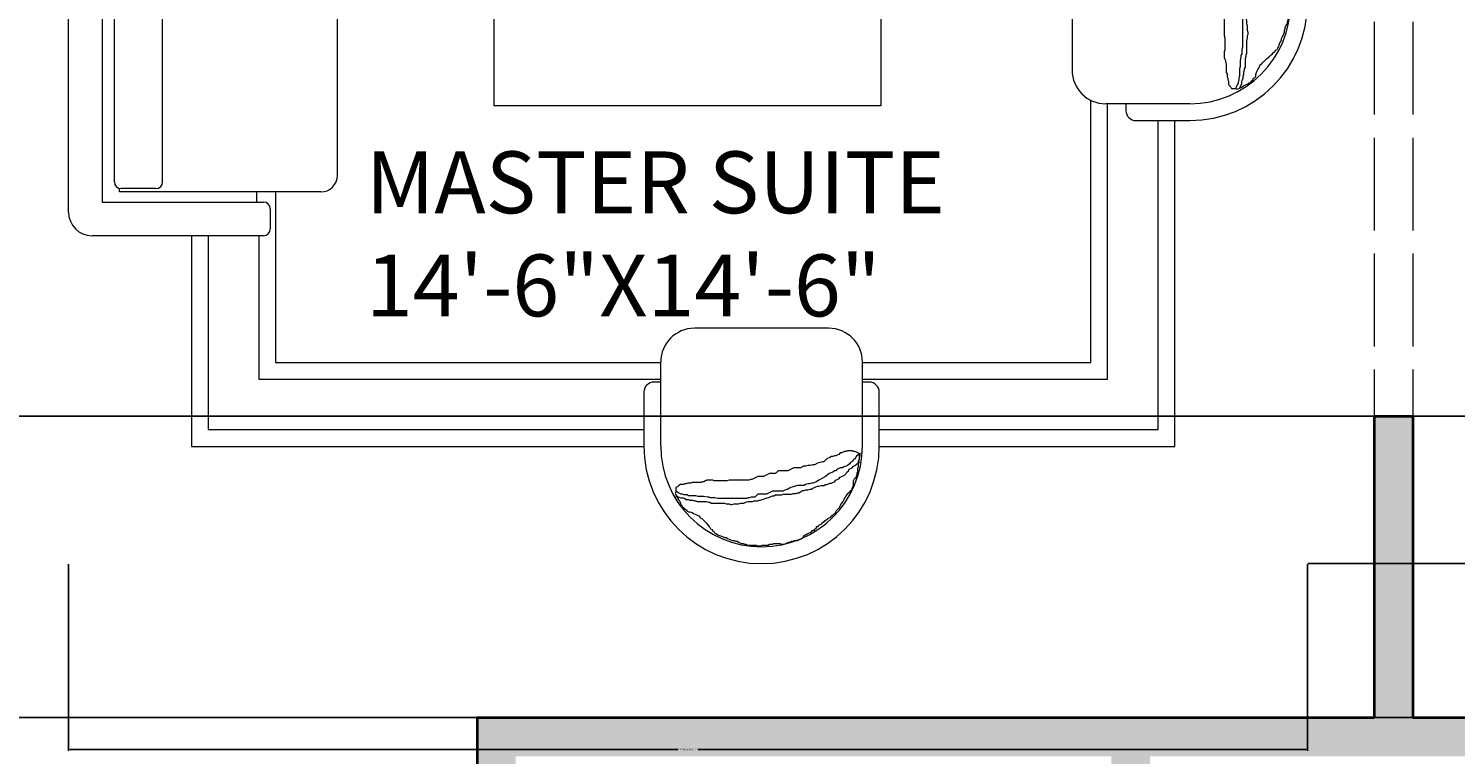
# Model space of a CAD drawing. Units: inches. Extents: x 2330 to 3943, y 1763 to 3461.
# Tile 28 of 40: x 3097 to 3281, y 2975 to 3069. Entities that reach past the tile are written whole.
import ezdxf

# ---------------------------------------------------------------- set-up
doc = ezdxf.new("R2010")
doc.units = ezdxf.units.IN
doc.linetypes.add('ACAD_ISO02W100', pattern=[15, 12, -3])
for name, color, linetype, lineweight in [('A-ANNO-DIMS', 2, 'Continuous', 18), ('A-AREA-IDEN', 7, 'Continuous', 18), ('A-FURN', 8, 'Continuous', 13), ('A-WALL', 7, 'Continuous', 40), ('A-WALL-OVHD', 7, 'ACAD_ISO02W100', 18), ('A-WALL-PATT', 252, 'Continuous', 13)]:
    doc.layers.add(name, color=color, linetype=linetype, lineweight=lineweight)
doc.styles.get("Standard").update_dxf_attribs({"font": 'arial.ttf'})
doc.dimstyles.get("Standard").update_dxf_attribs({"dimtxt": 0.18, "dimasz": 0.18, "dimexe": 0.18, "dimexo": 0.0625, "dimgap": 0.09, "dimtad": 0, "dimtih": 1, "dimtoh": 1, "dimdec": 4, "dimzin": 0, "dimdsep": 46, "dimtxsty": 'Standard', "dimcen": 0.09, "dimadec": 0, "dimazin": 0, "dimtfac": 1, "dimtdec": 4, "dimtofl": 0, "dimtmove": 0, "dimatfit": 3, "dimfxl": 1, "dimtolj": 1, "dimtzin": 0, "dimarcsym": 0})

# ---------------------------------------------------------------- blocks, each defined once
blk = doc.blocks.new('A$C78064EA7')
for p, q in [((932.1, 3320.6), (2792.1, 3320.6)), ((862.1, 2740.6), (862.1, 3250.6)), ((2862.1, 3250.6), (2862.1, 2740.6)), ((962.1, 3220.6), (962.1, 2740.6)), ((2762.1, 3220.6), (962.1, 3220.6)), ((1022.1, 3184.3), (1532.1, 3184.3)), ((1612.1, 3184.3), (2112.1, 3184.3)), ((2192.1, 3184.3), (2702.1, 3184.3)), ((2762.1, 2740.6), (2762.1, 3220.6)), ((469.8, 3064.3), (542.4, 3166)), ((476.1, 3059), (564.4, 3147.3)), ((992.1, 3168.5), (1002.1, 3168.5)), ((992.1, 2570.6), (992.1, 3168.5)), ((1002.1, 3060.6), (1002.1, 3164.3)), ((1551.6, 3168.5), (1562.1, 3168.5)), ((1552.1, 3060.6), (1552.1, 3164.3)), ((1562.1, 2570.6), (1562.1, 3168.5)), ((1582.1, 3168.5), (1592.5, 3168.5)), ((1582.1, 2570.6), (1582.1, 3168.5)), ((1592.1, 3060.6), (1592.1, 3164.3)), ((2131.6, 3168.5), (2142.1, 3168.5)), ((2132.1, 3060.6), (2132.1, 3164.3)), ((2142.1, 2570.6), (2142.1, 3168.5)), ((2162.1, 3168.5), (2172.5, 3168.5)), ((2162.1, 2570.6), (2162.1, 3168.5)), ((2172.1, 3060.6), (2172.1, 3164.3)), ((2721.6, 3168.5), (2732.1, 3168.5)), ((2722.1, 3060.6), (2722.1, 3164.3)), ((2732.1, 3168.5), (2732.1, 2570.6)), ((3248.1, 3059), (3159.7, 3147.3)), ((3254.4, 3064.3), (3181.7, 3166)), ((392.2, 3035.7), (270.9, 3066)), ((3331.9, 3035.7), (3453.2, 3066)), ((391.1, 3029.8), (267.1, 3045.3)), ((1022.1, 3040.6), (1532.1, 3040.6)), ((1612.1, 3040.6), (2112.1, 3040.6)), ((2192.1, 3040.6), (2702.1, 3040.6)), ((3333, 3029.8), (3457.1, 3045.3)), ((465.5, 2980.2), (527.5, 2871.7)), ((469.8, 2982.9), (542.4, 2881.2)), ((3254.4, 2982.9), (3181.7, 2881.2)), ((3258.6, 2980.2), (3196.6, 2871.7)), ((862.1, 2823.6), (765.7, 2823.6)), ((2958.4, 2823.6), (2862.1, 2823.6)), ((862.1, 2773.6), (765.7, 2773.6)), ((962.1, 2760.6), (992.1, 2760.6)), ((2732.1, 2760.6), (2762.1, 2760.6)), ((2958.4, 2773.6), (2862.1, 2773.6)), ((942.1, 2720.6), (882.1, 2720.6)), ((2842.1, 2720.6), (2782.1, 2720.6)), ((365.7, 2698.6), (365.7, 2405.5)), ((415.7, 2698.6), (415.7, 2405.5)), ((3240.7, 2017.9), (3240.7, 2698.6)), ((3290.7, 2017.9), (3290.7, 2698.6)), ((992.1, 2623.6), (560, 2623.6)), ((560, 2405.5), (560, 2623.6)), ((1562.1, 2600.6), (1582.1, 2600.6)), ((2142.1, 2600.6), (2162.1, 2600.6)), ((992.1, 2573.6), (615.7, 2573.6)), ((615.7, 2573.6), (615.7, 2275.5)), ((1042.1, 2520.6), (1512.1, 2520.6)), ((1632.1, 2520.6), (2092.1, 2520.6)), ((2212.1, 2520.6), (2682.1, 2520.6)), ((70, 2405.5), (580, 2405.5)), ((600, 2385.5), (600, 2325.5)), ((0, 1045.5), (0, 2335.5)), ((580, 2305.5), (100, 2305.5)), ((100, 2305.5), (100, 1075.5)), ((560, 2275.5), (560, 2305.5)), ((152.1, 2275.5), (750, 2275.5)), ((152.1, 2265.1), (152.1, 2275.5)), ((260, 2265.5), (156.3, 2265.5)), ((136.3, 1735.5), (136.3, 2245.5)), ((280, 1735.5), (280, 2245.5)), ((800, 1755.5), (800, 2225.5)), ((3335.1, 2017.9), (3175.1, 2017.9)), ((3335.1, 1967.9), (3085.1, 1967.9)), ((3145.1, 1987.9), (3145.1, 1967.9)), ((3358.2, 1958.7), (3353.6, 1950)), ((3358.2, 1961), (3355.9, 1961)), ((3362.5, 1958.7), (3358.2, 1961)), ((3362.5, 1961), (3358.2, 1958.7)), ((3358.2, 1958.7), (3362.5, 1954.4)), ((3366.8, 1961), (3362.5, 1961)), ((3375.5, 1958.7), (3362.5, 1958.7)), ((3362.5, 1954.4), (3364.5, 1950)), ((3380.1, 1956.4), (3375.5, 1958.7)), ((3397.4, 1956.4), (3380.1, 1956.4)), ((3384.4, 1958.7), (3382.1, 1958.7)), ((3386.4, 1954.4), (3384.4, 1958.7)), ((3388.7, 1950), (3386.4, 1954.4)), ((3402, 1954.4), (3397.4, 1956.4)), ((3410.6, 1954.4), (3402, 1954.4)), ((3415, 1952.1), (3410.6, 1954.4)), ((3351.6, 1941.1), (3349.3, 1936.8)), ((3349.3, 1936.8), (3349.3, 1923.5)), ((3349.3, 1923.5), (3351.6, 1919.2)), ((3353.6, 1950), (3351.6, 1945.4)), ((3351.6, 1945.4), (3351.6, 1941.1)), ((3351.6, 1919.2), (3351.6, 1914.9)), ((3351.6, 1914.9), (3353.6, 1910.5)), ((3353.6, 1910.5), (3355.9, 1906.2)), ((3364.5, 1950), (3369.1, 1947.7)), ((3369.1, 1947.7), (3373.5, 1945.4)), ((3373.5, 1945.4), (3375.5, 1941.1)), ((3375.5, 1941.1), (3380.1, 1939.1)), ((3380.1, 1939.1), (3384.4, 1932.4)), ((3384.4, 1932.4), (3388.7, 1928.1)), ((3393.1, 1945.4), (3388.7, 1950)), ((3388.7, 1928.1), (3393.1, 1923.5)), ((3395.4, 1941.1), (3393.1, 1945.4)), ((3393.1, 1923.5), (3395.4, 1919.2)), ((3399.7, 1936.8), (3395.4, 1941.1)), ((3395.4, 1919.2), (3397.4, 1912.5)), ((3397.4, 1912.5), (3399.7, 1908.2)), ((3402, 1932.4), (3399.7, 1936.8)), ((3404, 1928.1), (3402, 1932.4)), ((3408.6, 1925.8), (3404, 1928.1)), ((3412.9, 1921.5), (3408.6, 1925.8)), ((3417.3, 1919.2), (3412.9, 1921.5)), ((3419.6, 1952.1), (3415, 1952.1)), ((3421.6, 1914.9), (3417.3, 1919.2)), ((3423.9, 1950), (3419.6, 1952.1)), ((3423.9, 1910.5), (3421.6, 1914.9)), ((3428.2, 1950), (3423.9, 1950)), ((3425.9, 1906.2), (3423.9, 1910.5)), ((3430.5, 1945.4), (3428.2, 1950)), ((3434.8, 1943.4), (3430.5, 1945.4)), ((3439.2, 1941.1), (3434.8, 1943.4)), ((3452.4, 1941.1), (3439.2, 1941.1)), ((3456.7, 1939.1), (3452.4, 1941.1)), ((3461.1, 1936.8), (3456.7, 1939.1)), ((3465.4, 1936.8), (3461.1, 1936.8)), ((3467.7, 1932.4), (3465.4, 1936.8)), ((3472, 1930.1), (3467.7, 1932.4)), ((3474.3, 1925.8), (3472, 1930.1)), ((3478.7, 1923.5), (3474.3, 1925.8)), ((3483, 1919.2), (3478.7, 1923.5)), ((3487.3, 1917.2), (3483, 1919.2)), ((3491.6, 1914.9), (3487.3, 1917.2)), ((3496.2, 1912.5), (3491.6, 1914.9)), ((3500.6, 1910.5), (3496.2, 1912.5)), ((3504.9, 1906.2), (3500.6, 1910.5)), ((2985.1, 1867.9), (2985.1, 1467.9)), ((3355.9, 1906.2), (3355.9, 1901.6)), ((3355.9, 1901.6), (3360.2, 1897.3)), ((3360.2, 1897.3), (3362.5, 1892.9)), ((3362.5, 1892.9), (3364.5, 1888.6)), ((3364.5, 1888.6), (3364.5, 1884.3)), ((3364.5, 1884.3), (3366.8, 1879.7)), ((3366.8, 1879.7), (3366.8, 1875.3)), ((3366.8, 1875.3), (3369.1, 1871)), ((3369.1, 1871), (3373.5, 1862.3)), ((3399.7, 1908.2), (3399.7, 1901.6)), ((3399.7, 1901.6), (3402, 1897.3)), ((3402, 1897.3), (3404, 1892.9)), ((3404, 1892.9), (3408.6, 1888.6)), ((3408.6, 1888.6), (3408.6, 1884.3)), ((3408.6, 1884.3), (3412.9, 1879.7)), ((3412.9, 1879.7), (3417.3, 1869)), ((3417.3, 1869), (3425.9, 1858)), ((3428.2, 1901.6), (3425.9, 1906.2)), ((3432.5, 1897.3), (3428.2, 1901.6)), ((3434.8, 1892.9), (3432.5, 1897.3)), ((3436.9, 1888.6), (3434.8, 1892.9)), ((3441.5, 1884.3), (3436.9, 1888.6)), ((3443.5, 1879.7), (3441.5, 1884.3)), ((3445.8, 1875.3), (3443.5, 1879.7)), ((3445.8, 1871), (3445.8, 1875.3)), ((3447.8, 1866.7), (3445.8, 1871)), ((3509.2, 1903.9), (3504.9, 1906.2)), ((3513.8, 1901.6), (3509.2, 1903.9)), ((3518.1, 1899.6), (3513.8, 1901.6)), ((3522.5, 1895.2), (3518.1, 1899.6)), ((3526.8, 1890.6), (3522.5, 1895.2)), ((3531.1, 1888.6), (3526.8, 1890.6)), ((3535.7, 1886.3), (3531.1, 1888.6)), ((3537.7, 1882), (3535.7, 1886.3)), ((3542.1, 1879.7), (3537.7, 1882)), ((3542.1, 1875.3), (3542.1, 1879.7)), ((3546.7, 1873.3), (3542.1, 1875.3)), ((3548.7, 1869), (3546.7, 1873.3)), ((3551, 1864.4), (3548.7, 1869)), ((3373.5, 1862.3), (3382.1, 1853.4)), ((3382.1, 1853.4), (3382.1, 1849.1)), ((3382.1, 1849.1), (3384.4, 1842.4)), ((3384.4, 1842.4), (3386.4, 1833.8)), ((3386.4, 1833.8), (3391, 1825.1)), ((3391, 1825.1), (3391, 1820.5)), ((3425.9, 1858), (3430.5, 1849.1)), ((3430.5, 1849.1), (3434.8, 1842.4)), ((3434.8, 1842.4), (3436.9, 1838.1)), ((3436.9, 1838.1), (3441.5, 1831.5)), ((3441.5, 1831.5), (3443.5, 1825.1)), ((3443.5, 1825.1), (3445.8, 1820.5)), ((3450.1, 1862.3), (3447.8, 1866.7)), ((3450.1, 1858), (3450.1, 1862.3)), ((3452.4, 1853.4), (3450.1, 1858)), ((3452.4, 1844.8), (3452.4, 1853.4)), ((3454.4, 1838.1), (3452.4, 1844.8)), ((3454.4, 1833.8), (3454.4, 1838.1)), ((3456.7, 1829.5), (3454.4, 1833.8)), ((3458.8, 1825.1), (3456.7, 1829.5)), ((3461.1, 1820.5), (3458.8, 1825.1)), ((3555.3, 1860), (3551, 1864.4)), ((3557.6, 1855.7), (3555.3, 1860)), ((3561.9, 1853.4), (3557.6, 1855.7)), ((3561.9, 1849.1), (3561.9, 1853.4)), ((3566.3, 1847.1), (3561.9, 1849.1)), ((3568.6, 1842.4), (3566.3, 1847.1)), ((3570.6, 1838.1), (3568.6, 1842.4)), ((3574.9, 1836.1), (3570.6, 1838.1)), ((3574.9, 1831.5), (3574.9, 1836.1)), ((3579.5, 1831.5), (3574.9, 1831.5)), ((3581.5, 1827.2), (3579.5, 1831.5)), ((3585.9, 1825.1), (3581.5, 1827.2)), ((3585.9, 1820.5), (3585.9, 1825.1)), ((3391, 1820.5), (3393.1, 1811.9)), ((3393.1, 1811.9), (3393.1, 1805.2)), ((3393.1, 1805.2), (3395.4, 1798.6)), ((3395.4, 1798.6), (3395.4, 1792.2)), ((3395.4, 1792.2), (3399.7, 1783.3)), ((3399.7, 1783.3), (3399.7, 1763.7)), ((3445.8, 1820.5), (3445.8, 1816.2)), ((3445.8, 1816.2), (3447.8, 1809.6)), ((3447.8, 1809.6), (3447.8, 1805.2)), ((3447.8, 1805.2), (3450.1, 1798.6)), ((3450.1, 1798.6), (3452.4, 1794.3)), ((3452.4, 1794.3), (3452.4, 1774.7)), ((3463.4, 1816.2), (3461.1, 1820.5)), ((3463.4, 1811.9), (3463.4, 1816.2)), ((3465.4, 1805.2), (3463.4, 1811.9)), ((3465.4, 1798.6), (3465.4, 1805.2)), ((3467.7, 1794.3), (3465.4, 1798.6)), ((3467.7, 1789.9), (3467.7, 1794.3)), ((3472, 1783.3), (3467.7, 1789.9)), ((3474.3, 1779), (3472, 1783.3)), ((3590.5, 1816.2), (3585.9, 1820.5)), ((3592.5, 1811.9), (3590.5, 1816.2)), ((3594.8, 1807.5), (3592.5, 1811.9)), ((3596.8, 1803.2), (3594.8, 1807.5)), ((3599.1, 1798.6), (3596.8, 1803.2)), ((3601.4, 1794.3), (3599.1, 1798.6)), ((3605.7, 1792.2), (3601.4, 1794.3)), ((3610.1, 1787.6), (3605.7, 1792.2)), ((3612.4, 1783.3), (3610.1, 1787.6)), ((3614.4, 1779), (3612.4, 1783.3)), ((3399.7, 1763.7), (3408.6, 1746.1)), ((3408.6, 1746.1), (3408.6, 1717.5)), ((3452.4, 1774.7), (3454.4, 1768)), ((3454.4, 1768), (3456.7, 1761.4)), ((3456.7, 1761.4), (3458.8, 1755)), ((3458.8, 1755), (3461.1, 1750.4)), ((3461.1, 1750.4), (3463.4, 1746.1)), ((3463.4, 1746.1), (3465.4, 1739.5)), ((3474.3, 1774.7), (3474.3, 1779)), ((3476.3, 1770.3), (3474.3, 1774.7)), ((3476.3, 1761.4), (3476.3, 1770.3)), ((3478.7, 1757.1), (3476.3, 1761.4)), ((3478.7, 1733.1), (3478.7, 1757.1)), ((3616.7, 1774.7), (3614.4, 1779)), ((3616.7, 1766), (3616.7, 1774.7)), ((3618.7, 1761.4), (3616.7, 1766)), ((3618.7, 1757.1), (3618.7, 1761.4)), ((3621, 1752.7), (3618.7, 1757.1)), ((3621, 1748.4), (3621, 1752.7)), ((3623.3, 1744.1), (3621, 1748.4)), ((3625.3, 1739.5), (3623.3, 1744.1)), ((152.1, 1705.5), (152.1, 1716)), ((750, 1705.5), (152.1, 1705.5)), ((260, 1715.5), (156.3, 1715.5)), ((720, 1685.5), (720, 1705.5)), ((3408.6, 1717.5), (3417.3, 1708.9)), ((3417.3, 1708.9), (3417.3, 1691.3)), ((3465.4, 1739.5), (3467.7, 1735.1)), ((3467.7, 1735.1), (3469.7, 1730.8)), ((3469.7, 1730.8), (3469.7, 1700.2)), ((3469.7, 1700.2), (3478.7, 1682.6)), ((3480.7, 1728.5), (3478.7, 1733.1)), ((3480.7, 1708.9), (3480.7, 1728.5)), ((3483, 1704.6), (3480.7, 1708.9)), ((3483, 1700.2), (3483, 1704.6)), ((3485.3, 1695.6), (3483, 1700.2)), ((3627.6, 1735.1), (3625.3, 1739.5)), ((3625.3, 1722.1), (3627.6, 1726.5)), ((3625.3, 1704.6), (3625.3, 1722.1)), ((3627.6, 1700.2), (3625.3, 1704.6)), ((3627.6, 1726.5), (3627.6, 1735.1)), ((3627.6, 1691.3), (3627.6, 1700.2)), ((750, 1675.5), (152.1, 1675.5)), ((152.1, 1665.1), (152.1, 1675.5)), ((260, 1665.5), (156.3, 1665.5)), ((720, 1675.5), (720, 1695.5)), ((3417.3, 1691.3), (3425.9, 1674)), ((3425.9, 1674), (3425.9, 1656.4)), ((3425.9, 1656.4), (3434.8, 1638.8)), ((3478.7, 1682.6), (3478.7, 1656.4)), ((3478.7, 1656.4), (3487.3, 1647.4)), ((3487.3, 1691.3), (3485.3, 1695.6)), ((3491.6, 1678.3), (3487.3, 1691.3)), ((3493.9, 1669.4), (3491.6, 1678.3)), ((3496.2, 1665), (3493.9, 1669.4)), ((3496.2, 1660.7), (3496.2, 1665)), ((3498.2, 1656.4), (3496.2, 1660.7)), ((3498.2, 1645.4), (3498.2, 1656.4)), ((3629.9, 1687), (3627.6, 1691.3)), ((3629.9, 1669.4), (3629.9, 1687)), ((3632, 1665), (3629.9, 1669.4)), ((3629.9, 1652), (3632, 1656.4)), ((3632, 1656.4), (3632, 1665)), ((136.3, 1135.5), (136.3, 1645.5)), ((280, 1135.5), (280, 1645.5)), ((800, 1155.5), (800, 1625.5)), ((3434.8, 1638.8), (3434.8, 1634.5)), ((3434.8, 1634.5), (3436.9, 1630.1)), ((3436.9, 1630.1), (3436.9, 1571)), ((3487.3, 1647.4), (3487.3, 1636.5)), ((3487.3, 1636.5), (3489.6, 1632.1)), ((3489.6, 1632.1), (3489.6, 1627.8)), ((3489.6, 1627.8), (3491.6, 1623.5)), ((3491.6, 1623.5), (3491.6, 1538.1)), ((3500.6, 1641.1), (3498.2, 1645.4)), ((3500.6, 1627.8), (3500.6, 1641.1)), ((3502.6, 1621.2), (3500.6, 1627.8)), ((3504.9, 1614.5), (3502.6, 1621.2)), ((3504.9, 1605.9), (3504.9, 1614.5)), ((3625.3, 1612.5), (3627.6, 1616.9)), ((3627.6, 1621.2), (3629.9, 1625.5)), ((3627.6, 1616.9), (3627.6, 1621.2)), ((3629.9, 1625.5), (3629.9, 1652)), ((3436.9, 1571), (3439.2, 1564.4)), ((3507.2, 1599.3), (3504.9, 1605.9)), ((3507.2, 1586.3), (3507.2, 1599.3)), ((3509.2, 1579.6), (3507.2, 1586.3)), ((3507.2, 1571), (3509.2, 1575.3)), ((3507.2, 1562), (3507.2, 1571)), ((3509.2, 1575.3), (3509.2, 1579.6)), ((3610.1, 1566.4), (3612.4, 1571)), ((3612.4, 1571), (3614.4, 1575.3)), ((3614.4, 1575.3), (3616.7, 1582)), ((3616.7, 1586.3), (3618.7, 1590.6)), ((3616.7, 1582), (3616.7, 1586.3)), ((3618.7, 1594.9), (3621, 1599.3)), ((3618.7, 1590.6), (3618.7, 1594.9)), ((3621, 1599.3), (3623.3, 1603.9)), ((3623.3, 1603.9), (3625.3, 1608.2)), ((3625.3, 1608.2), (3625.3, 1612.5)), ((3439.2, 1564.4), (3439.2, 1527.1)), ((3491.6, 1538.1), (3489.6, 1529.2)), ((3489.6, 1529.2), (3489.6, 1516.2)), ((3504.9, 1557.7), (3507.2, 1562)), ((3504.9, 1518.2), (3504.9, 1557.7)), ((3590.5, 1527.1), (3594.8, 1529.2)), ((3594.8, 1529.2), (3596.8, 1533.5)), ((3596.8, 1533.5), (3599.1, 1538.1)), ((3599.1, 1538.1), (3601.4, 1542.4)), ((3601.4, 1542.4), (3603.4, 1549.1)), ((3603.4, 1549.1), (3605.7, 1553.4)), ((3605.7, 1553.4), (3607.8, 1557.7)), ((3607.8, 1562), (3610.1, 1566.4)), ((3607.8, 1557.7), (3607.8, 1562)), ((3439.2, 1527.1), (3436.9, 1522.5)), ((3436.9, 1522.5), (3436.9, 1505.2)), ((3436.9, 1505.2), (3439.2, 1500.9)), ((3439.2, 1500.9), (3441.5, 1496.3)), ((3441.5, 1496.3), (3441.5, 1491.9)), ((3441.5, 1491.9), (3443.5, 1487.6)), ((3443.5, 1487.6), (3443.5, 1461.4)), ((3487.3, 1507.2), (3485.3, 1496.3)), ((3485.3, 1496.3), (3485.3, 1479)), ((3489.6, 1516.2), (3487.3, 1511.9)), ((3487.3, 1511.9), (3487.3, 1507.2)), ((3500.6, 1502.9), (3502.6, 1509.5)), ((3500.6, 1476.7), (3500.6, 1502.9)), ((3502.6, 1513.9), (3504.9, 1518.2)), ((3502.6, 1509.5), (3502.6, 1513.9)), ((3548.7, 1485.3), (3551, 1489.9)), ((3551, 1489.9), (3564, 1502.9)), ((3564, 1502.9), (3572.9, 1509.5)), ((3572.9, 1509.5), (3577.2, 1513.9)), ((3577.2, 1513.9), (3581.5, 1516.2)), ((3581.5, 1516.2), (3583.8, 1520.5)), ((3583.8, 1520.5), (3588.2, 1522.5)), ((3588.2, 1522.5), (3590.5, 1527.1)), ((3443.5, 1461.4), (3445.8, 1457)), ((3445.8, 1457), (3445.8, 1448.1)), ((3445.8, 1448.1), (3447.8, 1443.8)), ((3447.8, 1443.8), (3447.8, 1439.4)), ((3483, 1450.4), (3480.7, 1446.1)), ((3480.7, 1446.1), (3480.7, 1437.1)), ((3485.3, 1479), (3483, 1472.3)), ((3483, 1472.3), (3483, 1450.4)), ((3491.6, 1439.4), (3493.9, 1443.8)), ((3493.9, 1450.4), (3496.2, 1454.7)), ((3493.9, 1443.8), (3493.9, 1450.4)), ((3496.2, 1463.4), (3498.2, 1468)), ((3496.2, 1454.7), (3496.2, 1463.4)), ((3498.2, 1472.3), (3500.6, 1476.7)), ((3498.2, 1468), (3498.2, 1472.3)), ((3522.5, 1439.4), (3524.8, 1443.8)), ((3524.8, 1443.8), (3529.1, 1446.1)), ((3529.1, 1446.1), (3531.1, 1450.4)), ((3531.1, 1454.7), (3533.4, 1461.4)), ((3531.1, 1450.4), (3531.1, 1454.7)), ((3533.4, 1461.4), (3535.7, 1465.7)), ((3535.7, 1465.7), (3537.7, 1470)), ((3537.7, 1470), (3540, 1474.3)), ((3540, 1474.3), (3542.1, 1479)), ((3542.1, 1479), (3544.4, 1483.3)), ((3544.4, 1483.3), (3548.7, 1485.3)), ((3447.8, 1439.4), (3450.1, 1435.1)), ((3450.1, 1435.1), (3450.1, 1426.2)), ((3450.1, 1426.2), (3452.4, 1421.8)), ((3452.4, 1421.8), (3456.7, 1417.5)), ((3456.7, 1417.5), (3458.8, 1413.2)), ((3458.8, 1413.2), (3472, 1413.2)), ((3474.3, 1419.8), (3472, 1415.2)), ((3472, 1415.2), (3472, 1413.2)), ((3472, 1413.2), (3476.3, 1410.9)), ((3476.3, 1424.2), (3474.3, 1419.8)), ((3478.7, 1428.5), (3476.3, 1424.2)), ((3476.3, 1410.9), (3480.7, 1413.2)), ((3480.7, 1437.1), (3478.7, 1432.8)), ((3478.7, 1432.8), (3478.7, 1428.5)), ((3480.7, 1413.2), (3485.3, 1415.2)), ((3485.3, 1417.5), (3487.3, 1421.8)), ((3485.3, 1413.2), (3485.3, 1417.5)), ((3485.3, 1415.2), (3489.6, 1417.5)), ((3487.3, 1421.8), (3489.6, 1426.2)), ((3489.6, 1435.1), (3491.6, 1439.4)), ((3489.6, 1426.2), (3489.6, 1435.1)), ((3489.6, 1417.5), (3496.2, 1421.8)), ((3496.2, 1421.8), (3500.6, 1424.2)), ((3500.6, 1424.2), (3504.9, 1426.2)), ((3504.9, 1426.2), (3509.2, 1426.2)), ((3509.2, 1426.2), (3511.5, 1430.5)), ((3511.5, 1430.5), (3515.8, 1430.5)), ((3515.8, 1430.5), (3518.1, 1435.1)), ((3518.1, 1435.1), (3522.5, 1439.4)), ((3335.1, 1367.9), (3085.1, 1367.9)), ((3145.1, 1367.9), (3145.1, 1347.9)), ((3175.1, 1317.9), (3335.1, 1317.9)), ((152.1, 1105.5), (152.1, 1115.5)), ((750, 1105.5), (152.1, 1105.5)), ((260, 1115.5), (156.3, 1115.5)), ((560, 1075.5), (560, 1105.5)), ((100, 1075.5), (580, 1075.5)), ((600, 1055.5), (600, 995.5)), ((580, 975.5), (70, 975.5)), ((2261.5, 700), (1861.5, 700)), ((1761.5, 350), (1761.5, 600)), ((2361.5, 350), (2361.5, 600)), ((1711.5, 510), (1711.5, 350)), ((1761.5, 540), (1741.5, 540)), ((2381.5, 540), (2361.5, 540)), ((2411.5, 350), (2411.5, 510)), ((2227.4, 298.6), (2218.8, 294)), ((2236.1, 300.7), (2227.4, 298.6)), ((2242.7, 303), (2236.1, 300.7)), ((2247, 303), (2242.7, 303)), ((2256, 311.6), (2247, 303)), ((2264.6, 315.9), (2256, 311.6)), ((2269, 318.2), (2264.6, 315.9)), ((2273.3, 318.2), (2269, 318.2)), ((2277.9, 320.5), (2273.3, 318.2)), ((2282.2, 320.5), (2277.9, 320.5)), ((2286.6, 322.6), (2282.2, 320.5)), ((2290.9, 324.9), (2286.6, 322.6)), ((2295.2, 329.2), (2290.9, 324.9)), ((2299.8, 329.2), (2295.2, 329.2)), ((2304.2, 331.5), (2299.8, 329.2)), ((2308.5, 333.5), (2304.2, 331.5)), ((2312.8, 333.5), (2308.5, 333.5)), ((2317.1, 335.8), (2312.8, 333.5)), ((2330.4, 335.8), (2317.1, 335.8)), ((2326.1, 300.7), (2321.8, 296.3)), ((2332.7, 305), (2326.1, 300.7)), ((2334.7, 333.5), (2330.4, 335.8)), ((2334.7, 309.6), (2332.7, 305)), ((2339.1, 333.5), (2334.7, 333.5)), ((2339.1, 311.6), (2334.7, 309.6)), ((2343.7, 331.5), (2339.1, 333.5)), ((2341.4, 315.9), (2339.1, 311.6)), ((2343.7, 320.5), (2341.4, 315.9)), ((2352.3, 326.9), (2343.7, 331.5)), ((2348, 322.6), (2343.7, 320.5)), ((2343.7, 296.3), (2348, 298.6)), ((2352.3, 326.9), (2348, 322.6)), ((2348, 298.6), (2352.3, 300.7)), ((2350, 305), (2352.3, 309.6)), ((2350, 287.7), (2350, 305)), ((2352.3, 322.6), (2354.6, 326.9)), ((2354.6, 322.6), (2352.3, 326.9)), ((2352.3, 309.6), (2352.3, 322.6)), ((2352.3, 300.7), (2352.3, 303)), ((2354.6, 326.9), (2354.6, 329.2)), ((2354.6, 318.2), (2354.6, 322.6)), ((2050, 259.2), (2032.4, 250.2)), ((2067.6, 259.2), (2050, 259.2)), ((2084.9, 267.8), (2067.6, 259.2)), ((2102.5, 267.8), (2084.9, 267.8)), ((2111.2, 276.5), (2102.5, 267.8)), ((2139.7, 276.5), (2111.2, 276.5)), ((2157.3, 285.4), (2139.7, 276.5)), ((2176.9, 285.4), (2157.3, 285.4)), ((2185.9, 289.7), (2176.9, 285.4)), ((2192.2, 289.7), (2185.9, 289.7)), ((2198.9, 292), (2192.2, 289.7)), ((2205.5, 292), (2198.9, 292)), ((2214.2, 294), (2205.5, 292)), ((2218.8, 294), (2214.2, 294)), ((2251.7, 259.2), (2242.7, 254.6)), ((2262.6, 267.8), (2251.7, 259.2)), ((2273.3, 272.1), (2262.6, 267.8)), ((2277.9, 276.5), (2273.3, 272.1)), ((2282.2, 276.5), (2277.9, 276.5)), ((2286.6, 281.1), (2282.2, 276.5)), ((2290.9, 283.1), (2286.6, 281.1)), ((2295.2, 285.4), (2290.9, 283.1)), ((2290.9, 252.5), (2295.2, 256.9)), ((2301.9, 285.4), (2295.2, 285.4)), ((2295.2, 256.9), (2299.8, 259.2)), ((2299.8, 259.2), (2304.2, 261.2)), ((2306.2, 287.7), (2301.9, 285.4)), ((2304.2, 261.2), (2308.5, 263.5)), ((2312.8, 289.7), (2306.2, 287.7)), ((2308.5, 263.5), (2312.8, 267.8)), ((2317.1, 292), (2312.8, 289.7)), ((2312.8, 267.8), (2315.1, 272.1)), ((2315.1, 272.1), (2319.5, 276.5)), ((2321.8, 296.3), (2317.1, 292)), ((2319.5, 276.5), (2321.8, 281.1)), ((2321.8, 281.1), (2326.1, 283.1)), ((2326.1, 283.1), (2330.4, 285.4)), ((2330.4, 285.4), (2334.7, 289.7)), ((2334.7, 289.7), (2339.1, 292)), ((2339.1, 292), (2343.7, 296.3)), ((2339.1, 254.6), (2343.7, 256.9)), ((2343.7, 261.2), (2345.7, 265.5)), ((2343.7, 256.9), (2343.7, 261.2)), ((2345.7, 270.1), (2348, 274.4)), ((2345.7, 265.5), (2345.7, 270.1)), ((2348, 283.1), (2350, 287.7)), ((2348, 274.4), (2348, 283.1)), ((1806.8, 213.1), (1804.5, 208.7)), ((1811.2, 228.3), (1806.8, 226.3)), ((1806.8, 226.3), (1806.8, 213.1)), ((1808.9, 213.1), (1806.8, 213.1)), ((1813.5, 210.7), (1808.9, 213.1)), ((1815.5, 232.7), (1811.2, 228.3)), ((1819.8, 235), (1815.5, 232.7)), ((1828.8, 235), (1819.8, 235)), ((1833.1, 237.3), (1828.8, 235)), ((1837.4, 237.3), (1833.1, 237.3)), ((1841.7, 239.3), (1837.4, 237.3)), ((1850.7, 239.3), (1841.7, 239.3)), ((1855, 241.6), (1850.7, 239.3)), ((1881.3, 241.6), (1855, 241.6)), ((1885.6, 243.6), (1881.3, 241.6)), ((1889.9, 243.6), (1885.6, 243.6)), ((1894.5, 245.9), (1889.9, 243.6)), ((1898.9, 248.2), (1894.5, 245.9)), ((1916.2, 248.2), (1898.9, 248.2)), ((1920.8, 245.9), (1916.2, 248.2)), ((1958, 245.9), (1920.8, 245.9)), ((1964.6, 248.2), (1958, 245.9)), ((2023.8, 248.2), (1964.6, 248.2)), ((2028.1, 250.2), (2023.8, 248.2)), ((2032.4, 250.2), (2028.1, 250.2)), ((2093.9, 215.4), (2076.3, 206.4)), ((2124.4, 215.4), (2093.9, 215.4)), ((2128.8, 217.4), (2124.4, 215.4)), ((2133.1, 219.7), (2128.8, 217.4)), ((2139.7, 221.7), (2133.1, 219.7)), ((2144.1, 224), (2139.7, 221.7)), ((2148.7, 226.3), (2144.1, 224)), ((2155, 228.3), (2148.7, 226.3)), ((2161.7, 230.6), (2155, 228.3)), ((2168.3, 232.7), (2161.7, 230.6)), ((2187.9, 232.7), (2168.3, 232.7)), ((2172.6, 210.7), (2176.9, 213.1)), ((2176.9, 213.1), (2183.6, 217.4)), ((2183.6, 217.4), (2187.9, 217.4)), ((2192.2, 235), (2187.9, 232.7)), ((2187.9, 217.4), (2192.2, 219.7)), ((2198.9, 237.3), (2192.2, 235)), ((2192.2, 219.7), (2198.9, 219.7)), ((2203.2, 237.3), (2198.9, 237.3)), ((2198.9, 219.7), (2205.5, 221.7)), ((2209.8, 239.3), (2203.2, 237.3)), ((2205.5, 221.7), (2209.8, 221.7)), ((2214.2, 239.3), (2209.8, 239.3)), ((2209.8, 221.7), (2214.2, 224)), ((2218.8, 241.6), (2214.2, 239.3)), ((2214.2, 224), (2218.8, 226.3)), ((2225.1, 243.6), (2218.8, 241.6)), ((2218.8, 226.3), (2223.1, 228.3)), ((2223.1, 228.3), (2227.4, 230.6)), ((2231.8, 248.2), (2225.1, 243.6)), ((2227.4, 230.6), (2231.8, 230.6)), ((2236.1, 250.2), (2231.8, 248.2)), ((2231.8, 230.6), (2238.4, 232.7)), ((2242.7, 254.6), (2236.1, 250.2)), ((2238.4, 232.7), (2247, 232.7)), ((2247, 232.7), (2251.7, 235)), ((2251.7, 235), (2256, 235)), ((2256, 235), (2260.3, 237.3)), ((2260.3, 237.3), (2264.6, 239.3)), ((2264.6, 239.3), (2269, 239.3)), ((2269, 239.3), (2273.3, 241.6)), ((2273.3, 241.6), (2277.9, 243.6)), ((2277.9, 243.6), (2282.2, 248.2)), ((2282.2, 248.2), (2286.6, 250.2)), ((2286.6, 250.2), (2290.9, 252.5)), ((2319.5, 210.7), (2323.8, 213.1)), ((2323.8, 213.1), (2326.1, 217.4)), ((2326.1, 217.4), (2330.4, 219.7)), ((2330.4, 224), (2332.7, 228.3)), ((2330.4, 219.7), (2330.4, 224)), ((2332.7, 228.3), (2334.7, 232.7)), ((2334.7, 245.9), (2337.1, 250.2)), ((2334.7, 232.7), (2334.7, 245.9)), ((2337.1, 250.2), (2339.1, 254.6)), ((1804.5, 208.7), (1806.8, 204.4)), ((1806.8, 204.4), (1808.9, 199.8)), ((1806.8, 199.8), (1811.2, 199.8)), ((1808.9, 199.8), (1811.2, 195.5)), ((1811.2, 199.8), (1815.5, 197.8)), ((1811.2, 195.5), (1815.5, 188.8)), ((1817.8, 208.7), (1813.5, 210.7)), ((1815.5, 197.8), (1819.8, 195.5)), ((1815.5, 188.8), (1817.8, 184.5)), ((1822.1, 206.4), (1817.8, 208.7)), ((1817.8, 184.5), (1819.8, 180.2)), ((1819.8, 195.5), (1828.8, 195.5)), ((1819.8, 180.2), (1819.8, 175.9)), ((1819.8, 175.9), (1824.1, 173.6)), ((1826.5, 206.4), (1822.1, 206.4)), ((1824.1, 173.6), (1824.1, 169.2)), ((1830.8, 204.4), (1826.5, 206.4)), ((1828.8, 195.5), (1833.1, 193.5)), ((1839.7, 204.4), (1830.8, 204.4)), ((1833.1, 193.5), (1837.4, 191.2)), ((1837.4, 191.2), (1844, 191.2)), ((1844, 202.1), (1839.7, 204.4)), ((1866, 202.1), (1844, 202.1)), ((1844, 191.2), (1848.4, 188.8)), ((1848.4, 188.8), (1857, 188.8)), ((1857, 188.8), (1861.6, 186.8)), ((1861.6, 186.8), (1866, 186.8)), ((1872.6, 199.8), (1866, 202.1)), ((1866, 186.8), (1870.3, 184.5)), ((1870.3, 184.5), (1896.6, 184.5)), ((1889.9, 199.8), (1872.6, 199.8)), ((1900.9, 197.8), (1889.9, 199.8)), ((1896.6, 184.5), (1903.2, 182.5)), ((1905.5, 197.8), (1900.9, 197.8)), ((1903.2, 182.5), (1907.5, 182.5)), ((1909.8, 195.5), (1905.5, 197.8)), ((1907.5, 182.5), (1911.8, 180.2)), ((1922.8, 195.5), (1909.8, 195.5)), ((1911.8, 180.2), (1951.4, 180.2)), ((1931.7, 193.5), (1922.8, 195.5)), ((2017.1, 193.5), (1931.7, 193.5)), ((1951.4, 180.2), (1955.7, 177.9)), ((1955.7, 177.9), (1964.6, 177.9)), ((1964.6, 177.9), (1969, 175.9)), ((1969, 175.9), (1973.3, 175.9)), ((1973.3, 175.9), (1979.9, 177.9)), ((1979.9, 177.9), (1992.9, 177.9)), ((1992.9, 177.9), (1999.5, 180.2)), ((1999.5, 180.2), (2008.2, 180.2)), ((2008.2, 180.2), (2014.8, 182.5)), ((2014.8, 182.5), (2021.5, 184.5)), ((2021.5, 195.5), (2017.1, 193.5)), ((2025.8, 195.5), (2021.5, 195.5)), ((2021.5, 184.5), (2034.7, 184.5)), ((2030.1, 197.8), (2025.8, 195.5)), ((2041.1, 197.8), (2030.1, 197.8)), ((2034.7, 184.5), (2039.1, 186.8)), ((2039.1, 186.8), (2050, 186.8)), ((2050, 206.4), (2041.1, 197.8)), ((2076.3, 206.4), (2050, 206.4)), ((2050, 186.8), (2054.3, 188.8)), ((2054.3, 188.8), (2058.7, 188.8)), ((2058.7, 188.8), (2063, 191.2)), ((2063, 191.2), (2071.9, 193.5)), ((2071.9, 193.5), (2084.9, 197.8)), ((2084.9, 197.8), (2089.3, 199.8)), ((2089.3, 199.8), (2093.9, 202.1)), ((2093.9, 202.1), (2098.2, 202.1)), ((2098.2, 202.1), (2102.5, 204.4)), ((2102.5, 204.4), (2122.1, 204.4)), ((2122.1, 204.4), (2126.8, 206.4)), ((2126.8, 206.4), (2150.7, 206.4)), ((2150.7, 206.4), (2155, 208.7)), ((2155, 208.7), (2164, 208.7)), ((2164, 208.7), (2168.3, 210.7)), ((2168.3, 210.7), (2172.6, 210.7)), ((2293.2, 166.9), (2295.2, 171.3)), ((2295.2, 171.3), (2297.5, 175.9)), ((2297.5, 175.9), (2299.8, 180.2)), ((2299.8, 180.2), (2304.2, 184.5)), ((2304.2, 184.5), (2306.2, 188.8)), ((2306.2, 188.8), (2308.5, 193.5)), ((2308.5, 193.5), (2310.8, 197.8)), ((2310.8, 197.8), (2312.8, 202.1)), ((2312.8, 202.1), (2317.1, 206.4)), ((2317.1, 206.4), (2319.5, 210.7)), ((1824.1, 169.2), (1828.8, 166.9)), ((1828.8, 166.9), (1833.1, 162.6)), ((1833.1, 162.6), (1837.4, 160.3)), ((1837.4, 160.3), (1839.7, 156)), ((1839.7, 156), (1844, 154)), ((1844, 154), (1848.4, 154)), ((1848.4, 154), (1855, 151.7)), ((1855, 151.7), (1859.3, 149.4)), ((1859.3, 149.4), (1863.7, 147.3)), ((1863.7, 147.3), (1868, 145)), ((1868, 145), (1872.6, 143)), ((1872.6, 143), (1876.9, 140.7)), ((1876.9, 140.7), (1879, 136.4)), ((1879, 136.4), (1883.6, 134.1)), ((1883.6, 134.1), (1896.6, 121.1)), ((2247, 123.1), (2249.4, 127.5)), ((2249.4, 127.5), (2253.7, 129.8)), ((2253.7, 129.8), (2258, 134.1)), ((2258, 134.1), (2262.6, 136.4)), ((2262.6, 136.4), (2267, 138.4)), ((2267, 138.4), (2269, 143)), ((2269, 143), (2273.3, 143)), ((2273.3, 143), (2275.6, 147.3)), ((2275.6, 147.3), (2279.9, 149.4)), ((2279.9, 149.4), (2282.2, 154)), ((2282.2, 154), (2284.3, 158.3)), ((2284.3, 158.3), (2288.9, 162.6)), ((2288.9, 162.6), (2293.2, 166.9)), ((1896.6, 121.1), (1903.2, 112.2)), ((1903.2, 112.2), (1907.5, 107.9)), ((1907.5, 107.9), (1909.8, 103.5)), ((1909.8, 103.5), (1914.1, 101.2)), ((1914.1, 101.2), (1916.2, 96.9)), ((1916.2, 96.9), (1920.8, 94.6)), ((1920.8, 94.6), (1922.8, 90.3)), ((1922.8, 90.3), (1927.1, 88.3)), ((1927.1, 88.3), (1931.7, 86)), ((1931.7, 86), (1936.1, 83.7)), ((2187.9, 83.7), (2192.2, 86)), ((2192.2, 86), (2196.9, 88.3)), ((2196.9, 88.3), (2201.2, 90.3)), ((2201.2, 90.3), (2205.5, 92.6)), ((2205.5, 92.6), (2209.8, 94.6)), ((2209.8, 94.6), (2214.2, 99.2)), ((2214.2, 99.2), (2218.8, 99.2)), ((2218.8, 99.2), (2220.8, 103.5)), ((2220.8, 103.5), (2225.1, 105.6)), ((2225.1, 110.2), (2229.7, 110.2)), ((2225.1, 105.6), (2225.1, 110.2)), ((2229.7, 110.2), (2231.8, 114.5)), ((2231.8, 114.5), (2236.1, 116.5)), ((2236.1, 116.5), (2240.7, 118.8)), ((2240.7, 118.8), (2242.7, 123.1)), ((2242.7, 123.1), (2247, 123.1)), ((1936.1, 83.7), (1942.7, 81.6)), ((1942.7, 81.6), (1947, 79.3)), ((1947, 79.3), (1951.4, 77.3)), ((1951.4, 77.3), (1955.7, 77.3)), ((1955.7, 77.3), (1960, 75)), ((1960, 75), (1964.6, 72.7)), ((1964.6, 72.7), (1969, 70.7)), ((1969, 70.7), (1975.6, 68.4)), ((1975.6, 68.4), (1979.9, 68.4)), ((1979.9, 68.4), (1984.2, 66.4)), ((1984.2, 66.4), (1988.6, 66.4)), ((1988.6, 66.4), (1992.9, 64.1)), ((1992.9, 64.1), (1997.5, 61.8)), ((1997.5, 61.8), (2001.8, 59.7)), ((2001.8, 59.7), (2006.2, 59.7)), ((2006.2, 59.7), (2010.5, 57.4)), ((2010.5, 57.4), (2014.8, 57.4)), ((2014.8, 57.4), (2019.2, 55.1)), ((2019.2, 55.1), (2045.7, 55.1)), ((2045.7, 55.1), (2050, 53.1)), ((2050, 53.1), (2058.7, 53.1)), ((2058.7, 53.1), (2063, 55.1)), ((2063, 55.1), (2080.6, 55.1)), ((2080.6, 55.1), (2084.9, 57.4)), ((2084.9, 57.4), (2093.9, 57.4)), ((2093.9, 57.4), (2098.2, 59.7)), ((2098.2, 59.7), (2115.8, 59.7)), ((2115.8, 59.7), (2120.1, 57.4)), ((2120.1, 57.4), (2128.8, 57.4)), ((2128.8, 57.4), (2133.1, 59.7)), ((2133.1, 59.7), (2137.7, 61.8)), ((2137.7, 61.8), (2142, 64.1)), ((2142, 64.1), (2146.4, 64.1)), ((2146.4, 64.1), (2150.7, 66.4)), ((2150.7, 66.4), (2155, 66.4)), ((2155, 66.4), (2159.6, 68.4)), ((2159.6, 68.4), (2168.3, 68.4)), ((2168.3, 68.4), (2172.6, 70.7)), ((2172.6, 70.7), (2176.9, 72.7)), ((2176.9, 72.7), (2181.3, 75)), ((2181.3, 75), (2185.9, 79.3)), ((2185.9, 79.3), (2187.9, 83.7))]:
    blk.add_line(p, q)
for points in [[(765.7, 2698.6), (115.7, 2698.6), (115.7, 3348.6), (765.7, 3348.6)], [(2958.4, 2698.6), (3608.4, 2698.6), (3608.4, 3348.6), (2958.4, 3348.6)], [(1265.7, 1361.6), (1265.7, 2011.6), (2415.7, 2011.6), (2415.7, 1361.6)]]:
    blk.add_lwpolyline(points, close=True)
for points in [[(3090.7, 1967.9), (3090.7, 2623.6), (2732.1, 2623.6)], [(3040.7, 1957.5), (3040.7, 2573.6), (2732.1, 2573.6)], [(2361.5, 598.6), (3040.7, 598.6), (3040.7, 1378.2)], [(2361.5, 548.6), (3090.7, 548.6), (3090.7, 1367.9)], [(2411.5, 348.6), (3290.7, 348.6), (3290.7, 1317.9)], [(2411.5, 398.6), (3240.7, 398.6), (3240.7, 1317.9)], [(615.7, 1105.5), (615.7, 598.6), (1761.5, 598.6)], [(365.7, 975.5), (365.7, 348.6), (1711.5, 348.6)], [(415.7, 975.5), (415.7, 398.6), (1711.5, 398.6)], [(565.7, 975.5), (565.7, 548.6), (1761.5, 548.6)]]:
    blk.add_lwpolyline(points)
for centre, radius in [((440.7, 3023.6), 175), ((3283.4, 3023.6), 175), ((440.7, 3023.6), 50), ((3283.4, 3023.6), 50), ((440.7, 3023.6), 25), ((3283.4, 3023.6), 25)]:
    blk.add_circle(centre, radius)
for centre, radius, start, end in [((932.1, 3250.6), 70, 90, 180), ((2792.1, 3250.6), 70, 0, 90), ((1022.1, 3164.3), 20, 90, 180), ((1532.1, 3164.3), 20, 0, 90), ((1612.1, 3164.3), 20, 90, 180), ((2112.1, 3164.3), 20, 0, 90), ((2192.1, 3164.3), 20, 90, 180), ((2702.1, 3164.3), 20, 0, 90), ((1022.1, 3060.6), 20, 180, 270), ((1532.1, 3060.6), 20, 270, 0), ((1612.1, 3060.6), 20, 180, 270), ((2112.1, 3060.6), 20, 270, 0), ((2192.1, 3060.6), 20, 180, 270), ((2702.1, 3060.6), 20, 270, 0), ((882.1, 2740.6), 20, 180, 270), ((942.1, 2740.6), 20, 270, 0), ((2782.1, 2740.6), 20, 180, 270), ((2842.1, 2740.6), 20, 270, 0), ((1042.1, 2570.6), 50, 180, 270), ((1512.1, 2570.6), 50, 270, 0), ((1632.1, 2570.6), 50, 180, 270), ((2092.1, 2570.6), 50, 270, 0), ((2212.1, 2570.6), 50, 180, 270), ((2682.1, 2570.6), 50, 270, 0), ((70, 2335.5), 70, 90, 180), ((580, 2385.5), 20, 0, 90), ((580, 2325.5), 20, 270, 0), ((156.3, 2245.5), 20, 90, 180), ((260, 2245.5), 20, 0, 90), ((750, 2225.5), 50, 0, 90), ((3175.1, 1987.9), 30, 90, 180), ((3335.1, 1667.9), 350, 270, 90), ((3085.1, 1867.9), 100, 90, 180), ((3335.1, 1667.9), 300, 270, 90), ((750, 1755.5), 50, 270, 0), ((156.3, 1735.5), 20, 180, 270), ((260, 1735.5), 20, 270, 0), ((156.3, 1645.5), 20, 90, 180), ((260, 1645.5), 20, 0, 90), ((750, 1625.5), 50, 0, 90), ((3085.1, 1467.9), 100, 180, 270), ((3175.1, 1347.9), 30, 180, 270), ((750, 1155.5), 50, 270, 0), ((156.3, 1135.5), 20, 180, 270), ((260, 1135.5), 20, 270, 0), ((580, 1055.5), 20, 0, 90), ((70, 1045.5), 70, 180, 270), ((580, 995.5), 20, 270, 0), ((1861.5, 600), 100, 90, 180), ((2261.5, 600), 100, 0, 90), ((1741.5, 510), 30, 90, 180), ((2381.5, 510), 30, 0, 90), ((2061.5, 350), 350, 180, 0), ((2061.5, 350), 300, 180, 360)]:
    blk.add_arc(centre, radius, start, end)
blk = doc.blocks.new('*D47')
at = {"layer": 'A-ANNO-DIMS', "color": 0, "lineweight": -2, "transparency": 16777216}
for p, q in [((3101.83, 2999.5), (3101.83, 2975.35)), ((3262.04, 2999.5), (3262.04, 2975.35)), ((3102.01, 2975.53), (3180.66, 2975.53)), ((3261.86, 2975.53), (3183.22, 2975.53))]:
    blk.add_line(p, q, dxfattribs=at)
at = {"layer": 'A-ANNO-DIMS', "color": 0, "transparency": 16777216}
for points in [[(3102.01, 2975.56), (3102.01, 2975.5), (3101.83, 2975.53)], [(3261.86, 2975.56), (3261.86, 2975.5), (3262.04, 2975.53)]]:
    blk.add_solid(points, dxfattribs=at)
at = {"layer": 'Defpoints', "color": 0, "transparency": 16777216}
for p in [(3101.83, 2999.57), (3262.04, 2999.57), (3262.04, 2975.53)]:
    blk.add_point(p, dxfattribs=at)
at = {"layer": 'A-ANNO-DIMS', "color": 0, "transparency": 16777216, "insert": (3181.94, 2975.53), "char_height": 0.18, "attachment_point": 5}
blk.add_mtext('\\A1;SUITE SEATING 160', dxfattribs=at)
blk = doc.blocks.new('*D48')
at = {"layer": 'A-ANNO-DIMS', "color": 0, "lineweight": -2, "transparency": 16777216}
for p, q in [((3262.1, 3145.15), (3286.25, 3145.15)), ((3286.07, 3144.97), (3286.07, 3072.54)), ((3286.07, 2999.75), (3286.07, 3072.18)), ((3262.1, 2999.57), (3286.25, 2999.57))]:
    blk.add_line(p, q, dxfattribs=at)
at = {"layer": 'A-ANNO-DIMS', "color": 0, "transparency": 16777216}
for points in [[(3286.04, 3144.97), (3286.1, 3144.97), (3286.07, 3145.15)], [(3286.04, 2999.75), (3286.1, 2999.75), (3286.07, 2999.57)]]:
    blk.add_solid(points, dxfattribs=at)
at = {"layer": 'Defpoints', "color": 0, "transparency": 16777216}
for p in [(3262.04, 3145.15), (3286.07, 3145.15), (3262.04, 2999.57)]:
    blk.add_point(p, dxfattribs=at)
at = {"layer": 'A-ANNO-DIMS', "color": 0, "transparency": 16777216, "insert": (3286.07, 3072.36), "char_height": 0.18, "attachment_point": 5}
blk.add_mtext('\\A1;146', dxfattribs=at)
blk = doc.blocks.new('*D93')
at = {"layer": 'A-ANNO-DIMS', "color": 0, "lineweight": -2, "transparency": 16777216}
for p, q in [((3446.6, 3018.65), (2330.5, 3018.65)), ((2330.68, 3018.47), (2330.68, 2999.33)), ((2330.68, 2979.83), (2330.68, 2998.97)), ((3446.6, 2979.65), (2330.5, 2979.65))]:
    blk.add_line(p, q, dxfattribs=at)
at = {"layer": 'A-ANNO-DIMS', "color": 0, "transparency": 16777216}
for points in [[(2330.65, 3018.47), (2330.71, 3018.47), (2330.68, 3018.65)], [(2330.65, 2979.83), (2330.71, 2979.83), (2330.68, 2979.65)]]:
    blk.add_solid(points, dxfattribs=at)
at = {"layer": 'Defpoints', "color": 0, "transparency": 16777216}
for p in [(2330.68, 3018.65), (3446.66, 3018.65), (3446.66, 2979.65)]:
    blk.add_point(p, dxfattribs=at)
at = {"layer": 'A-ANNO-DIMS', "color": 0, "transparency": 16777216, "insert": (2330.68, 2999.15), "char_height": 0.18, "attachment_point": 5}
blk.add_mtext('\\A1;39', dxfattribs=at)

msp = doc.modelspace()

# ---------------------------------------------------------------- hatches: boundary and pattern name
at = {"layer": 'A-WALL-PATT'}
h = msp.add_hatch(color=256, dxfattribs=at)
h.dxf.hatch_style = 1
h.paths.add_polyline_path([(3241.6605, 2974.6524), (3376.7746, 2974.6524, -0.16828569), (3398.3014, 2935.4254), (3407.174, 2936.9344, 0.12044914), (3392.5913, 2970.6524), (3455.6605, 2970.6524), (3455.6605, 3018.6524), (3446.6605, 3018.6524), (3446.6605, 2979.6524), (3275.6605, 2979.6524), (3275.6605, 3018.6524), (3270.6605, 3018.6524), (3270.6605, 2979.6524), (3154.6605, 2979.6524), (3154.6605, 2918.1524), (3150.6605, 2918.1524), (3150.6605, 2913.1524), (3154.6605, 2913.1524), (3154.6605, 2863.6524), (3159.6605, 2863.6524), (3159.6605, 2867.6524), (3196.6605, 2867.6524), (3196.6605, 2872.6524), (3159.6605, 2872.6524), (3159.6605, 2974.6524), (3236.6605, 2974.6524), (3236.6605, 2906.6524), (3241.6605, 2906.6524)])

# ---------------------------------------------------------------- linework, layer by layer
at = {"layer": 'A-WALL'}
for p, q in [((3270.6605, 3018.6524), (3275.6605, 3018.6524)), ((3270.6605, 3018.6524), (3270.6605, 2979.6524)), ((3275.6605, 3018.6524), (3275.6605, 2979.6524)), ((3154.6605, 2979.6524), (3270.6605, 2979.6524)), ((3154.6605, 2979.6524), (3154.6605, 2918.1524)), ((3275.6605, 2979.6524), (3446.6605, 2979.6524))]:
    msp.add_line(p, q, dxfattribs=at)
at = {"layer": 'A-WALL-OVHD'}
for p, q in [((3270.6605, 3114.6524), (3270.6605, 3018.6524)), ((3275.6605, 3114.6524), (3275.6605, 3018.6524))]:
    msp.add_line(p, q, dxfattribs=at)

# ---------------------------------------------------------------- block references
at = {"layer": 'A-FURN', "xscale": 0.0434754410177484, "yscale": 0.0434754410177484, "zscale": 0.0434754410177484}
msp.add_blockref('A$C78064EA7', (3101.8308, 2999.5664), dxfattribs=at)

# ---------------------------------------------------------------- texts
at = {"layer": 'A-AREA-IDEN', "insert": (3140.2855, 3052.879), "char_height": 8, "attachment_point": 1}
msp.add_mtext_dynamic_manual_height_columns('MASTER SUITE\\P14\'-6"X14\'-6"', width=95.491359, gutter_width=12.5, heights=[0], dxfattribs=at)

# ---------------------------------------------------------------- dimensions: what is measured, and where the dimension line sits
at = {"layer": 'A-ANNO-DIMS'}
for base, p1, p2, picture, middle in [((3286.0727, 3145.1485), (3262.0412, 2999.5664), (3262.0412, 3145.1485), '*D48', (3286.0727, 3072.3575)), ((2330.6824, 3018.6524), (3446.6605, 2979.6524), (3446.6605, 3018.6524), '*D93', (2330.6824, 2999.1524))]:
    dim = msp.add_linear_dim(base=base, p1=p1, p2=p2, angle=90, dimstyle='Standard', override={"dimdec": 0, "dimlfac": 1, "dimrnd": 0, "dimzin": 0, "dimdsep": 46, "dimlunit": 2}, dxfattribs=at)
    dim.commit()
    dim.dimension.update_dxf_attribs({"geometry": picture, "text_midpoint": middle})
dim = msp.add_linear_dim(base=(3262.0412, 2975.5349), p1=(3101.8308, 2999.5664), p2=(3262.0412, 2999.5664), text='SUITE SEATING <>', dimstyle='Standard', override={"dimdec": 0, "dimlfac": 1, "dimrnd": 0, "dimzin": 0, "dimdsep": 46, "dimlunit": 2}, dxfattribs=at)
dim.commit()
dim.dimension.update_dxf_attribs({"geometry": '*D47', "text_midpoint": (3181.936, 2975.5349)})

doc.saveas('drawing.dxf')
